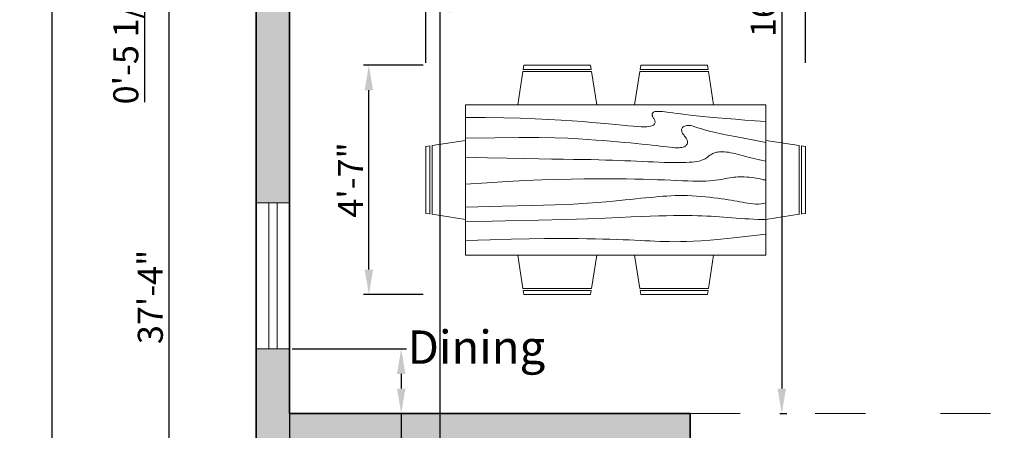
# Model space of a CAD drawing. Units: inches. Extents: x 2129 to 3258, y 1851 to 3021.
# Tile 5 of 10: x 2129 to 2365, y 2151 to 2250. Entities that reach past the tile are written whole.
import ezdxf

# ---------------------------------------------------------------- set-up
doc = ezdxf.new("R2010")
doc.units = ezdxf.units.IN
doc.linetypes.add('ACAD_ISO03W100', pattern=[30, 12, -18])
for name, color, linetype, lineweight in [('A-ANNO-DIMS', 2, 'Continuous', 18), ('A-AREA-IDEN', 7, 'Continuous', 20), ('A-FURN', 8, 'Continuous', 18), ('A-GLAZ', 4, 'Continuous', 18), ('A-WALL', 7, 'Continuous', 35), ('A-WALL-OVHD', 8, 'ACAD_ISO03W100', 18)]:
    doc.layers.add(name, color=color, linetype=linetype, lineweight=lineweight)
doc.layers.add('A-WALL-PATT', color=32, linetype='Continuous', lineweight=13, true_color=0xcd6928)
doc.styles.get("Standard").update_dxf_attribs({"font": 'arial.ttf'})
doc.dimstyles.new('ISO-25', dxfattribs={"dimtxt": 6, "dimasz": 6, "dimexe": 1.25, "dimexo": 0.625, "dimtad": 1, "dimdec": 1, "dimlunit": 3, "dimtxsty": 'Standard', "dimcen": 2.5, "dimclrd": 5, "dimclre": 5, "dimadec": 0, "dimazin": 0, "dimtfac": 1, "dimtdec": 1, "dimtmove": 0, "dimatfit": 3, "dimfxl": 1, "dimarcsym": 0})

# ---------------------------------------------------------------- blocks, each defined once
blk = doc.blocks.new('Dining Set - 36 x 72 in.')
for p, q in [((-22.2343, 26.00059), (-23.4847, 17.99762)), ((-22.2304, 26), (-5.7608, 26)), ((-22, 27.5), (-22.1562, 26.50042)), ((-5.8416, 26.5), (-22.1534, 26.5)), ((-22, 27.5), (-6, 27.5)), ((-5.8437, 26.49966), (-6, 27.5)), ((-4.5152, 17.99762), (-5.7655, 25.99926)), ((5.7657, 26.00059), (4.5153, 17.99762)), ((5.7696, 26), (22.2392, 26)), ((6, 27.5), (5.8438, 26.50042)), ((22.1584, 26.5), (5.8466, 26.5)), ((6, 27.5), (22, 27.5)), ((22.1563, 26.49966), (22, 27.5)), ((23.4848, 17.99762), (22.2345, 25.99926)), ((36, 18), (-36, 18)), ((-36, 18), (-36, -18)), ((36, -18), (36, 18)), ((-44.0006, 8.23428), (-35.9976, 9.48474)), ((44.0006, 8.23428), (35.9976, 9.48474)), ((-45.5, 8), (-44.5004, 8.15617)), ((-45.5, 8), (-45.5, -8)), ((-44.5, -8.15843), (-44.5, 8.15338)), ((-44, 8.23041), (-44, -8.23915)), ((44, 8.23041), (44, -8.23915)), ((44.5, -8.15843), (44.5, 8.15338)), ((45.5, 8), (44.5005, 8.15617)), ((45.5, 8), (45.5, -8)), ((-44.4997, -8.15631), (-45.5, -8)), ((-35.9976, -9.48476), (-43.9993, -8.2345)), ((35.9976, -9.48476), (43.9993, -8.2345)), ((44.4997, -8.15631), (45.5, -8)), ((-36, -18), (36, -18)), ((-22.2343, -26.0006), (-23.4847, -17.99762)), ((-4.5152, -17.99762), (-5.7655, -25.99928)), ((5.7657, -26.0006), (4.5153, -17.99762)), ((23.4848, -17.99762), (22.2345, -25.99928)), ((-22.2304, -26), (-5.7608, -26)), ((-22, -27.5), (-22.1562, -26.50044)), ((-5.8416, -26.5), (-22.1534, -26.5)), ((-22, -27.5), (-6, -27.5)), ((-5.8437, -26.49967), (-6, -27.5)), ((5.7696, -26), (22.2392, -26)), ((6, -27.5), (5.8438, -26.50044)), ((22.1584, -26.5), (5.8466, -26.5)), ((6, -27.5), (22, -27.5)), ((22.1563, -26.49967), (22, -27.5))]:
    blk.add_line(p, q)
for points in [[(-36, 15), (-31.1772, 14.97754), (-26.8079, 14.91406), (-22.8538, 14.81543), (-19.276, 14.6875), (-16.0362, 14.53613), (-13.0957, 14.36718), (-10.4159, 14.18652), (-7.9583, 14), (-5.6904, 13.81315), (-3.6035, 13.63021), (-1.6954, 13.45508), (0.0365, 13.29166), (1.5945, 13.14388), (2.9811, 13.01562), (4.1988, 12.9108), (5.25, 12.83333), (6.1393, 12.78613), (6.8802, 12.76823), (7.4883, 12.77767), (7.9792, 12.8125), (8.3685, 12.87077), (8.6719, 12.95052), (8.9049, 13.0498), (9.0833, 13.16666), (9.2205, 13.29899), (9.3216, 13.44401), (9.3895, 13.59879), (9.4271, 13.76041), (9.4373, 13.92594), (9.4232, 14.09245), (9.3875, 14.257), (9.3333, 14.41666), (9.2638, 14.56917), (9.1836, 14.71484), (9.0975, 14.85465), (9.0104, 14.98958), (8.9272, 15.1206), (8.8529, 15.2487), (8.7922, 15.37483), (8.75, 15.5), (8.7305, 15.62467), (8.7344, 15.74739), (8.7617, 15.86621), (8.8125, 15.97916), (8.8867, 16.08431), (8.9844, 16.17968), (9.1055, 16.26334), (9.25, 16.33333), (9.4189, 16.38802), (9.6172, 16.42708), (9.8506, 16.45052), (10.125, 16.45833), (10.4463, 16.45052), (10.8203, 16.42708), (11.2529, 16.38802), (11.75, 16.33333), (12.3184, 16.26318), (12.9694, 16.17838), (13.7151, 16.07991), (14.5677, 15.96875), (15.5395, 15.84586), (16.6426, 15.71224), (17.8893, 15.56884), (19.2917, 15.41666), (20.859, 15.25667), (22.5879, 15.08984), (24.4721, 14.91715), (26.5052, 14.73958), (28.6809, 14.5581), (30.9929, 14.3737), (33.4347, 14.18733), (36, 14)], [(-36, 10), (-28.9766, 10.14274), (-23.1725, 10.20442), (-18.4241, 10.19775), (-14.5677, 10.13541), (-11.4399, 10.03011), (-8.877, 9.89453), (-6.7154, 9.74137), (-4.7917, 9.58333), (-2.9698, 9.43082), (-1.2246, 9.28515), (0.4415, 9.14534), (2.026, 9.01041), (3.5266, 8.87939), (4.9408, 8.7513), (6.266, 8.62516), (7.5, 8.5), (8.6411, 8.37549), (9.6914, 8.2539), (10.6538, 8.13818), (11.5312, 8.03125), (12.3267, 7.93603), (13.043, 7.85547), (13.6831, 7.79248), (14.25, 7.75), (14.7471, 7.7303), (15.1797, 7.73307), (15.5537, 7.75732), (15.875, 7.80208), (16.1494, 7.86637), (16.3828, 7.94922), (16.5811, 8.04964), (16.75, 8.16666), (16.8944, 8.29915), (17.0143, 8.44531), (17.1089, 8.60319), (17.1771, 8.77083), (17.218, 8.94629), (17.2305, 9.1276), (17.2137, 9.31282), (17.1667, 9.5), (17.0895, 9.6875), (16.987, 9.875), (16.8649, 10.0625), (16.7292, 10.25), (16.5856, 10.4375), (16.4401, 10.625), (16.2985, 10.8125), (16.1667, 11), (16.05, 11.18733), (15.9518, 11.3737), (15.8752, 11.5581), (15.8229, 11.73958), (15.798, 11.91715), (15.8034, 12.08984), (15.842, 12.25667), (15.9167, 12.41666), (16.0295, 12.56836), (16.1784, 12.70833), (16.3605, 12.83268), (16.5729, 12.9375), (16.8127, 13.01888), (17.0768, 13.07291), (17.3625, 13.0957), (17.6667, 13.08333), (17.9894, 13.03312), (18.3418, 12.94726), (18.7382, 12.82918), (19.1927, 12.68229), (19.7195, 12.51001), (20.3327, 12.31575), (21.0465, 12.10294), (21.875, 11.875), (22.8357, 11.63354), (23.959, 11.37304), (25.2786, 11.08618), (26.8282, 10.76562), (28.6414, 10.40405), (30.752, 9.99414), (33.1936, 9.52856), (36, 9)], [(-36, 5.5), (-30.7157, 5.3348), (-26.069, 5.20963), (-21.9946, 5.11767), (-18.4271, 5.05208), (-15.3009, 5.00602), (-12.5508, 4.97265), (-10.1112, 4.94515), (-7.9167, 4.91666), (-5.909, 4.88167), (-4.0586, 4.83984), (-2.3429, 4.79215), (-0.7396, 4.73958), (0.7739, 4.6831), (2.22, 4.6237), (3.6213, 4.56233), (5, 4.5), (6.373, 4.43782), (7.7344, 4.3776), (9.0723, 4.32129), (10.375, 4.27083), (11.6309, 4.22819), (12.8281, 4.19531), (13.9551, 4.17415), (15, 4.16666), (15.954, 4.17448), (16.819, 4.19791), (17.6001, 4.23698), (18.3021, 4.29166), (18.9299, 4.36198), (19.4883, 4.44791), (19.9823, 4.54948), (20.4167, 4.66666), (20.7969, 4.79899), (21.1302, 4.94401), (21.4245, 5.09879), (21.6875, 5.26041), (21.9271, 5.42594), (22.1511, 5.59245), (22.3672, 5.757), (22.5834, 5.91666), (22.8065, 6.06868), (23.0404, 6.21093), (23.2879, 6.34147), (23.5521, 6.45833), (23.8358, 6.55957), (24.142, 6.64323), (24.4735, 6.70735), (24.8334, 6.75), (25.2235, 6.76969), (25.642, 6.76692), (26.0858, 6.74267), (26.5521, 6.69791), (27.0379, 6.63362), (27.5404, 6.55078), (28.0565, 6.45036), (28.5834, 6.33333), (29.1242, 6.19987), (29.7071, 6.04687), (30.3661, 5.87044), (31.1354, 5.66666), (32.0493, 5.43164), (33.142, 5.16146), (34.4475, 4.85221), (36, 4.5)], [(-36, -1), (-30.7915, -0.6591), (-26.0195, -0.38216), (-21.6519, -0.16284), (-17.6563, 0.00521), (-14.0005, 0.12833), (-10.6523, 0.21289), (-7.5796, 0.26522), (-4.75, 0.29166), (-2.134, 0.29793), (0.2878, 0.28711), (2.5317, 0.26163), (4.6146, 0.22396), (6.5529, 0.17651), (8.3633, 0.12174), (10.0623, 0.06209), (11.6667, 0), (13.1899, -0.06201), (14.6341, -0.1211), (15.9982, -0.17432), (17.2813, -0.21875), (18.4823, -0.25147), (19.6003, -0.26953), (20.6343, -0.27002), (21.5834, -0.25), (22.4481, -0.20768), (23.2357, -0.14584), (23.9549, -0.06836), (24.6146, 0.02083), (25.2235, 0.11784), (25.7904, 0.21875), (26.3241, 0.31966), (26.8334, 0.41666), (27.3265, 0.50618), (27.8099, 0.58593), (28.2894, 0.65397), (28.7709, 0.70833), (29.2601, 0.74707), (29.763, 0.76823), (30.2855, 0.76985), (30.8334, 0.75), (31.4088, 0.70784), (31.9994, 0.64713), (32.589, 0.57275), (33.1615, 0.48958), (33.7008, 0.4025), (34.1908, 0.3164), (34.6153, 0.23616), (34.9584, 0.16666), (35.2099, 0.11165), (35.3848, 0.07031), (35.504, 0.04069), (35.5886, 0.02083), (35.6594, 0.00879), (35.7377, 0.0026), (35.8442, 0.00032), (36, 0)], [(-36, -6.5), (-27.1843, -6.31267), (-20.084, -6.1263), (-14.469, -5.9419), (-10.1094, -5.76042), (-6.7752, -5.58285), (-4.2363, -5.41016), (-2.2629, -5.24333), (-0.625, -5.08334), (0.8708, -4.93099), (2.2715, -4.78646), (3.5872, -4.64974), (4.8281, -4.52084), (6.0046, -4.39974), (7.127, -4.28646), (8.2053, -4.18099), (9.25, -4.08334), (10.2705, -3.99382), (11.2734, -3.91407), (12.2647, -3.84603), (13.25, -3.79167), (14.2354, -3.75293), (15.2266, -3.73177), (16.2295, -3.73015), (17.25, -3.75), (18.2912, -3.79248), (19.3451, -3.85547), (20.4009, -3.93604), (21.4479, -4.03125), (22.4754, -4.13819), (23.4727, -4.25391), (24.4289, -4.37549), (25.3334, -4.5), (26.1785, -4.62492), (26.9694, -4.74935), (27.7145, -4.87281), (28.4219, -4.99479), (29.1, -5.11483), (29.7572, -5.23242), (30.4016, -5.34709), (31.0417, -5.45834), (31.6837, -5.56437), (32.3262, -5.65821), (32.9658, -5.73153), (33.599, -5.77604), (34.2224, -5.78345), (34.8327, -5.74545), (35.4264, -5.65373), (36, -5.5)], [(-36, -10), (-26.4022, -9.81299), (-18.4675, -9.62891), (-11.9839, -9.45069), (-6.7396, -9.28125), (-2.5226, -9.12354), (0.8789, -8.98047), (3.6769, -8.85498), (6.0833, -8.75), (8.2767, -8.66765), (10.3021, -8.60677), (12.1712, -8.56543), (13.8958, -8.54167), (15.4876, -8.53353), (16.9583, -8.53907), (18.3197, -8.55632), (19.5834, -8.58334), (20.7616, -8.61841), (21.8685, -8.66081), (22.9188, -8.71004), (23.9271, -8.76563), (24.9081, -8.82707), (25.8763, -8.89388), (26.8465, -8.96558), (27.8334, -9.04167), (28.8474, -9.12118), (29.8828, -9.20117), (30.93, -9.27824), (31.9792, -9.34896), (33.0205, -9.40991), (34.0443, -9.45768), (35.0407, -9.48885), (36, -9.5)], [(-36, -14.5), (-30.0881, -14.33513), (-25.0332, -14.21224), (-20.7312, -14.12647), (-17.0781, -14.07292), (-13.97, -14.04671), (-11.3027, -14.04297), (-8.9724, -14.05681), (-6.875, -14.08334), (-4.9224, -14.11833), (-3.0905, -14.16016), (-1.3709, -14.20785), (0.2448, -14.26042), (1.7647, -14.3169), (3.1973, -14.3763), (4.5507, -14.43767), (5.8333, -14.5), (7.0554, -14.5621), (8.235, -14.62175), (9.3922, -14.67652), (10.5469, -14.72396), (11.7192, -14.76164), (12.929, -14.78711), (14.1965, -14.79794), (15.5417, -14.79167), (16.9933, -14.76424), (18.6152, -14.70508), (20.4804, -14.60197), (22.6615, -14.44271), (25.2312, -14.21509), (28.2624, -13.9069), (31.8277, -13.50594), (36, -13)]]:
    blk.add_lwpolyline(points)
blk = doc.blocks.new('*D5')
at = {"layer": 'A-ANNO-DIMS', "color": 0, "lineweight": -2, "transparency": 16777216}
for p, q in [((2185.3, 2407.23), (2163.77, 2407.23)), ((2165.02, 2401.23), (2165.02, 1965.23)), ((2185.3, 1959.23), (2163.77, 1959.23))]:
    blk.add_line(p, q, dxfattribs=at)
at = {"layer": 'A-ANNO-DIMS', "color": 0, "transparency": 16777216}
for points in [[(2164.02, 2401.23), (2166.02, 2401.23), (2165.02, 2407.23)], [(2164.02, 1965.23), (2166.02, 1965.23), (2165.02, 1959.23)]]:
    blk.add_solid(points, dxfattribs=at)
at = {"layer": 'Defpoints', "color": 0, "transparency": 16777216}
for p in [(2185.93, 2407.23), (2165.02, 1959.23), (2185.93, 1959.23)]:
    blk.add_point(p, dxfattribs=at)
at = {"layer": 'A-ANNO-DIMS', "color": 0, "transparency": 16777216, "insert": (2161.33, 2183.23), "char_height": 6, "attachment_point": 5, "rotation": 90}
blk.add_mtext('37\'-4"', dxfattribs=at)
blk = doc.blocks.new('*D6')
at = {"layer": 'A-ANNO-DIMS', "color": 0, "lineweight": -2, "transparency": 16777216}
for p, q in [((2185.3, 2407.23), (2135.71, 2407.23)), ((2136.96, 2401.23), (2136.96, 1885.23)), ((2185.3, 1879.23), (2135.71, 1879.23))]:
    blk.add_line(p, q, dxfattribs=at)
at = {"layer": 'A-ANNO-DIMS', "color": 0, "transparency": 16777216}
for points in [[(2135.96, 2401.23), (2137.96, 2401.23), (2136.96, 2407.23)], [(2135.96, 1885.23), (2137.96, 1885.23), (2136.96, 1879.23)]]:
    blk.add_solid(points, dxfattribs=at)
at = {"layer": 'Defpoints', "color": 0, "transparency": 16777216}
for p in [(2185.93, 2407.23), (2136.96, 1879.23), (2185.93, 1879.23)]:
    blk.add_point(p, dxfattribs=at)
at = {"layer": 'A-ANNO-DIMS', "color": 0, "transparency": 16777216, "insert": (2133.34, 2143.23), "char_height": 6, "attachment_point": 5, "rotation": 90}
blk.add_mtext("44'", dxfattribs=at)
blk = doc.blocks.new('*D7')
at = {"layer": 'A-ANNO-DIMS', "color": 0, "lineweight": -2, "transparency": 16777216}
for p, q in [((2311.4, 2347.23), (2313.14, 2347.23)), ((2311.89, 2341.23), (2311.89, 2161.23)), ((2311.4, 2155.23), (2313.14, 2155.23))]:
    blk.add_line(p, q, dxfattribs=at)
at = {"layer": 'A-ANNO-DIMS', "color": 0, "transparency": 16777216}
for points in [[(2310.89, 2341.23), (2312.89, 2341.23), (2311.89, 2347.23)], [(2310.89, 2161.23), (2312.89, 2161.23), (2311.89, 2155.23)]]:
    blk.add_solid(points, dxfattribs=at)
at = {"layer": 'Defpoints', "color": 0, "transparency": 16777216}
for p in [(2310.77, 2347.23), (2310.77, 2155.23), (2311.89, 2155.23)]:
    blk.add_point(p, dxfattribs=at)
at = {"layer": 'A-ANNO-DIMS', "color": 0, "transparency": 16777216, "insert": (2308.2, 2251.23), "char_height": 6, "attachment_point": 5, "rotation": 90}
blk.add_mtext("16'", dxfattribs=at)
blk = doc.blocks.new('WIN-PLAN-35')
for p, q in [((0, 5), (35, 5)), ((0, 3), (35, 3))]:
    blk.add_line(p, q)
blk.add_lwpolyline([(0, 8), (35, 8), (35, 0), (0, 0)], close=True)
blk = doc.blocks.new('*D78')
at = {"layer": 'A-ANNO-DIMS', "color": 5, "lineweight": -2, "transparency": 16777216}
for p, q in [((2226.58, 2239.39), (2226.58, 2253.67)), ((2317.58, 2239.39), (2317.58, 2253.67)), ((2232.58, 2252.42), (2311.58, 2252.42))]:
    blk.add_line(p, q, dxfattribs=at)
at = {"layer": 'A-ANNO-DIMS', "color": 5, "transparency": 16777216}
for points in [[(2232.58, 2253.42), (2232.58, 2251.42), (2226.58, 2252.42)], [(2311.58, 2253.42), (2311.58, 2251.42), (2317.58, 2252.42)]]:
    blk.add_solid(points, dxfattribs=at)
at = {"layer": 'Defpoints', "color": 0, "transparency": 16777216}
for p in [(2317.58, 2252.42), (2226.58, 2238.77), (2317.58, 2238.77)]:
    blk.add_point(p, dxfattribs=at)
at = {"layer": 'A-ANNO-DIMS', "color": 0, "transparency": 16777216, "insert": (2272.08, 2256.15), "char_height": 6, "attachment_point": 5}
blk.add_mtext('DINING SET 7\'-7"', dxfattribs=at)
blk = doc.blocks.new('*D79')
at = {"layer": 'A-ANNO-DIMS', "color": 5, "lineweight": -2, "transparency": 16777216}
for p, q in [((2225.95, 2238.77), (2211.68, 2238.77)), ((2212.93, 2189.77), (2212.93, 2232.77)), ((2225.95, 2183.77), (2211.68, 2183.77))]:
    blk.add_line(p, q, dxfattribs=at)
at = {"layer": 'A-ANNO-DIMS', "color": 5, "transparency": 16777216}
for points in [[(2211.93, 2232.77), (2213.93, 2232.77), (2212.93, 2238.77)], [(2211.93, 2189.77), (2213.93, 2189.77), (2212.93, 2183.77)]]:
    blk.add_solid(points, dxfattribs=at)
at = {"layer": 'Defpoints', "color": 0, "transparency": 16777216}
for p in [(2212.93, 2238.77), (2226.58, 2238.77), (2226.58, 2183.77)]:
    blk.add_point(p, dxfattribs=at)
at = {"layer": 'A-ANNO-DIMS', "color": 0, "transparency": 16777216, "insert": (2209.3, 2211.27), "char_height": 6, "attachment_point": 5, "rotation": 90}
blk.add_mtext('4\'-7"', dxfattribs=at)
blk = doc.blocks.new('*D97')
at = {"layer": 'A-ANNO-DIMS', "color": 5, "lineweight": -2, "transparency": 16777216}
for p, q in [((2193.93, 2272.48), (2193.93, 1851.23)), ((2229.93, 2272.48), (2229.93, 1851.23)), ((2199.93, 1852.48), (2223.93, 1852.48))]:
    blk.add_line(p, q, dxfattribs=at)
at = {"layer": 'A-ANNO-DIMS', "color": 5, "transparency": 16777216}
for points in [[(2199.93, 1853.48), (2199.93, 1851.48), (2193.93, 1852.48)], [(2223.93, 1853.48), (2223.93, 1851.48), (2229.93, 1852.48)]]:
    blk.add_solid(points, dxfattribs=at)
at = {"layer": 'Defpoints', "color": 0, "transparency": 16777216}
for p in [(2193.93, 2273.1), (2229.93, 2273.1), (2229.93, 1852.48)]:
    blk.add_point(p, dxfattribs=at)
at = {"layer": 'A-ANNO-DIMS', "color": 0, "transparency": 16777216, "insert": (2211.93, 1856.18), "char_height": 6, "attachment_point": 5}
blk.add_mtext('3\'-0"', dxfattribs=at)
blk = doc.blocks.new('*D106')
at = {"layer": 'A-ANNO-DIMS', "color": 5, "lineweight": -2, "transparency": 16777216}
for p, q in [((2159.18, 2284.42), (2159.18, 2290.42)), ((2207.23, 2278.42), (2157.93, 2278.42)), ((2159.18, 2278.42), (2159.18, 2273.1)), ((2193.3, 2273.1), (2157.93, 2273.1)), ((2159.18, 2267.1), (2159.18, 2229.92))]:
    blk.add_line(p, q, dxfattribs=at)
at = {"layer": 'A-ANNO-DIMS', "color": 5, "transparency": 16777216}
for points in [[(2158.18, 2284.42), (2160.18, 2284.42), (2159.18, 2278.42)], [(2158.18, 2267.1), (2160.18, 2267.1), (2159.18, 2273.1)]]:
    blk.add_solid(points, dxfattribs=at)
at = {"layer": 'Defpoints', "color": 0, "transparency": 16777216}
for p in [(2207.85, 2278.42), (2159.18, 2273.1), (2193.93, 2273.1)]:
    blk.add_point(p, dxfattribs=at)
at = {"layer": 'A-ANNO-DIMS', "color": 0, "transparency": 16777216, "insert": (2155.45, 2245.51), "char_height": 6, "attachment_point": 5, "rotation": 90}
blk.add_mtext('0\'-5 1/2"', dxfattribs=at)
blk = doc.blocks.new('*D110')
at = {"layer": 'A-ANNO-DIMS', "color": 5, "lineweight": -2, "transparency": 16777216}
for p, q in [((2194.55, 2170.77), (2221.93, 2170.77)), ((2220.68, 2164.77), (2220.68, 2161.23)), ((2194.55, 2155.23), (2221.93, 2155.23)), ((2220.68, 2155.23), (2220.68, 2118.62))]:
    blk.add_line(p, q, dxfattribs=at)
at = {"layer": 'A-ANNO-DIMS', "color": 5, "transparency": 16777216}
for points in [[(2219.68, 2164.77), (2221.68, 2164.77), (2220.68, 2170.77)], [(2219.68, 2161.23), (2221.68, 2161.23), (2220.68, 2155.23)]]:
    blk.add_solid(points, dxfattribs=at)
at = {"layer": 'Defpoints', "color": 0, "transparency": 16777216}
for p in [(2193.93, 2170.77), (2193.93, 2155.23), (2220.68, 2155.23)]:
    blk.add_point(p, dxfattribs=at)
at = {"layer": 'A-ANNO-DIMS', "color": 0, "transparency": 16777216, "insert": (2216.95, 2133.93), "char_height": 6, "attachment_point": 5, "rotation": 90}
blk.add_mtext('1\'-3 1/2"', dxfattribs=at)

msp = doc.modelspace()

# ---------------------------------------------------------------- hatches: boundary and pattern name
at = {"layer": 'A-WALL-PATT'}
h = msp.add_hatch(color=256, dxfattribs=at)
h.dxf.hatch_style = 1
h.paths.add_polyline_path([(2393.39, 2407.23), (2185.93, 2407.23), (2185.93, 2394.06), (2193.93, 2394.06), (2193.93, 2399.23), (2361.93, 2399.23), (2361.93, 2355.23), (2361.93, 2347.23), (2361.93, 2258.25), (2369.93, 2258.25), (2369.93, 2307.23), (2429.93, 2307.23), (2429.93, 2303.23), (2437.93, 2303.23), (2437.93, 2327.23), (2429.93, 2327.23), (2429.93, 2315.23), (2369.93, 2315.23), (2369.93, 2399.23), (2393.39, 2399.23)])
h.paths.add_polyline_path([(2569.93, 2407.23), (2410.42, 2407.23), (2410.42, 2399.23), (2429.93, 2399.23), (2429.93, 2351.23), (2437.93, 2351.23), (2437.93, 2399.23), (2561.93, 2399.23), (2561.93, 2317.22), (2569.93, 2317.22)])
h.paths.add_polyline_path([(2569.93, 2282.22), (2561.93, 2282.22), (2561.93, 2243.23), (2437.93, 2243.23), (2437.93, 2249.23), (2429.93, 2249.23), (2429.93, 2235.23), (2561.93, 2235.23), (2561.93, 2155.23), (2379.93, 2155.23), (2379.93, 2147.23), (2385.93, 2147.23), (2385.93, 2141.23), (2393.93, 2141.23), (2393.93, 2147.23), (2469.93, 2147.23), (2469.93, 2111.23), (2477.93, 2111.23), (2477.93, 2147.23), (2561.93, 2147.23), (2561.93, 2129.53), (2569.93, 2129.53)])
h.paths.add_polyline_path([(2569.93, 2112.5), (2561.93, 2112.5), (2561.93, 2063.23), (2477.93, 2063.23), (2477.93, 2069.23), (2469.93, 2069.23), (2469.93, 2063.23), (2445.93, 2063.23), (2445.93, 2055.23), (2561.93, 2055.23), (2561.93, 1951.04), (2569.93, 1951.04)])
h.paths.add_polyline_path([(2569.93, 1916.04), (2561.93, 1916.04), (2561.93, 1887.23), (2393.93, 1887.23), (2393.93, 2055.23), (2399.93, 2055.23), (2399.93, 2063.23), (2393.93, 2063.23), (2393.93, 2087.23), (2385.93, 2087.23), (2385.93, 1887.23), (2385.93, 1879.23), (2569.93, 1879.23)])
h.paths.add_polyline_path([(2193.93, 2147.23), (2289.93, 2147.23), (2289.93, 2155.23), (2193.93, 2155.23), (2193.93, 2170.77), (2185.93, 2170.77), (2185.93, 2056.85), (2193.93, 2056.85)])
h.paths.add_polyline_path([(2193.93, 2021.85), (2185.93, 2021.85), (2185.93, 1959.23), (2222.56, 1959.23), (2222.56, 1967.23), (2193.93, 1967.23)])
h.paths.add_polyline_path([(2307.93, 1967.23), (2257.56, 1967.23), (2257.56, 1959.23), (2307.93, 1959.23)])
h.paths.add_polyline_path([(2255.61, 2368.18), (2321.09, 2368.18), (2321.09, 2384.66), (2255.61, 2384.66)], flags=25)
h.paths.add_polyline_path([(2282.89, 2032.34), (2325.27, 2032.34), (2325.27, 2051.27), (2282.89, 2051.27)], flags=9)
h.paths.add_polyline_path([(2404.09, 1945.18), (2463.36, 1945.18), (2463.36, 1961.66), (2404.09, 1961.66)], flags=25)
h.paths.add_polyline_path([(2494.41, 2286.84), (2553.68, 2286.84), (2553.68, 2303.32), (2494.41, 2303.32)], flags=9)
h.paths.add_polyline_path([(2389.71, 2321.98), (2411.09, 2321.98), (2411.09, 2338.47), (2389.71, 2338.47)], flags=25)
h.paths.add_polyline_path([(2219.41, 2162.82), (2258.18, 2162.82), (2258.18, 2179.3), (2219.41, 2179.3)], flags=9)
h.paths.add_polyline_path([(2249.68, 2306.23), (2298.12, 2306.23), (2298.12, 2323.98), (2249.68, 2323.98)], flags=25)
h = msp.add_hatch(color=256, dxfattribs=at)
h.dxf.hatch_style = 1
h.paths.add_polyline_path([(2193.93, 2288.35), (2185.93, 2288.35), (2185.93, 2205.77), (2193.93, 2205.77)])
h.paths.add_polyline_path([(2193.93, 2347.23), (2310.77, 2347.23), (2310.77, 2355.23), (2193.93, 2355.23), (2193.93, 2359.06), (2185.93, 2359.06), (2185.93, 2323.35), (2193.93, 2323.35)])
h.paths.add_polyline_path([(2314.44, 2244.01), (2314.44, 2257.94), (2302.07, 2257.94), (2302.07, 2244.01)], flags=9)
h.paths.add_polyline_path([(2255.61, 2368.18), (2321.09, 2368.18), (2321.09, 2384.66), (2255.61, 2384.66)], flags=9)
h.paths.add_polyline_path([(2282.89, 2032.34), (2325.27, 2032.34), (2325.27, 2051.27), (2282.89, 2051.27)], flags=9)
h.paths.add_polyline_path([(2404.09, 1945.18), (2463.36, 1945.18), (2463.36, 1961.66), (2404.09, 1961.66)], flags=9)
h.paths.add_polyline_path([(2494.41, 2286.84), (2553.68, 2286.84), (2553.68, 2303.32), (2494.41, 2303.32)], flags=9)
h.paths.add_polyline_path([(2389.71, 2321.98), (2411.09, 2321.98), (2411.09, 2338.47), (2389.71, 2338.47)], flags=9)
h.paths.add_polyline_path([(2219.41, 2162.82), (2258.18, 2162.82), (2258.18, 2179.3), (2219.41, 2179.3)], flags=9)
h.paths.add_polyline_path([(2249.68, 2306.23), (2298.12, 2306.23), (2298.12, 2323.98), (2249.68, 2323.98)], flags=9)

# ---------------------------------------------------------------- linework, layer by layer
at = {"layer": 'A-WALL'}
for p in [(2193.93, 2155.23), (2289.93, 2147.23)]:
    msp.add_line(p, (2289.93, 2155.23), dxfattribs=at)
msp.add_lwpolyline([(2185.93, 2407.23), (2569.93, 2407.23), (2569.93, 1879.23), (2185.93, 1879.23)], close=True, dxfattribs=at)
msp.add_lwpolyline([(2193.93, 2155.23), (2193.93, 2347.23)], dxfattribs=at)
at = {"layer": 'A-WALL-OVHD'}
msp.add_line((2289.93, 2155.23), (2379.93, 2155.23), dxfattribs=at)

# ---------------------------------------------------------------- block references
at = {"layer": 'A-FURN'}
msp.add_blockref('Dining Set - 36 x 72 in.', (2272.08, 2211.27), dxfattribs=at)
at = {"layer": 'A-GLAZ', "rotation": 270.0000000000013}
msp.add_blockref('WIN-PLAN-35', (2185.93, 2205.77), dxfattribs=at)

# ---------------------------------------------------------------- texts
at = {"layer": 'A-AREA-IDEN', "insert": (2222.22, 2175.18), "char_height": 8, "attachment_point": 1}
msp.add_mtext_dynamic_manual_height_columns('{\\fArial|b1|i0|c0|p34;Dining}', width=32.1489, gutter_width=12.5, heights=[6.02], dxfattribs=at)

# ---------------------------------------------------------------- dimensions: what is measured, and where the dimension line sits
at = {"layer": 'A-ANNO-DIMS'}
for base, p1, p2, angle, override, picture, middle in [((2136.96, 1879.23), (2185.93, 2407.23), (2185.93, 1879.23), 90, {"dimclrd": 0, "dimclre": 0, "dimclrt": 0}, '*D6', (2133.34, 2143.23)), ((2165.02, 1959.23), (2185.93, 2407.23), (2185.93, 1959.23), 90, {"dimclrd": 0, "dimclre": 0, "dimclrt": 0}, '*D5', (2161.33, 2183.23)), ((2311.89, 2155.23), (2310.77, 2347.23), (2310.77, 2155.23), 90, {"dimclrd": 0, "dimclre": 0, "dimclrt": 0}, '*D7', (2308.2, 2251.23)), ((2159.18, 2273.1), (2207.85, 2278.42), (2193.93, 2273.1), 90, {"dimdec": 1, "dimlfac": 1, "dimrnd": 0, "dimzin": 1, "dimdsep": 46, "dimlunit": 4, "dimfrac": 2}, '*D106', (2155.45, 2245.51)), ((2212.93, 2238.77), (2226.58, 2183.77), (2226.58, 2238.77), 90, {"dimdec": 1, "dimlfac": 1, "dimrnd": 0, "dimzin": 1, "dimdsep": 46, "dimlunit": 4, "dimfrac": 2}, '*D79', (2209.3, 2211.27)), ((2220.68, 2155.23), (2193.93, 2170.77), (2193.93, 2155.23), 270, {"dimdec": 1, "dimlfac": 1, "dimrnd": 0, "dimzin": 1, "dimdsep": 46, "dimlunit": 4, "dimfrac": 2}, '*D110', (2216.95, 2133.93))]:
    dim = msp.add_linear_dim(base=base, p1=p1, p2=p2, angle=angle, dimstyle='ISO-25', override=override, dxfattribs=at)
    dim.commit()
    dim.dimension.update_dxf_attribs({"geometry": picture, "text_midpoint": middle})
dim = msp.add_linear_dim(base=(2229.93, 1852.48), p1=(2193.93, 2273.1), p2=(2229.93, 2273.1), dimstyle='ISO-25', override={"dimdec": 1, "dimlfac": 1, "dimrnd": 0, "dimzin": 1, "dimdsep": 46, "dimlunit": 4, "dimfrac": 2}, dxfattribs=at)
dim.commit()
dim.dimension.update_dxf_attribs({"geometry": '*D97', "text_midpoint": (2211.93, 1856.18)})
dim = msp.add_linear_dim(base=(2317.58, 2252.42), p1=(2226.58, 2238.77), p2=(2317.58, 2238.77), text='DINING SET <>', dimstyle='ISO-25', override={"dimdec": 1, "dimlfac": 1, "dimrnd": 0, "dimzin": 1, "dimdsep": 46, "dimlunit": 4, "dimfrac": 2}, dxfattribs=at)
dim.commit()
dim.dimension.update_dxf_attribs({"geometry": '*D78', "text_midpoint": (2272.08, 2256.15)})

doc.saveas('drawing.dxf')
